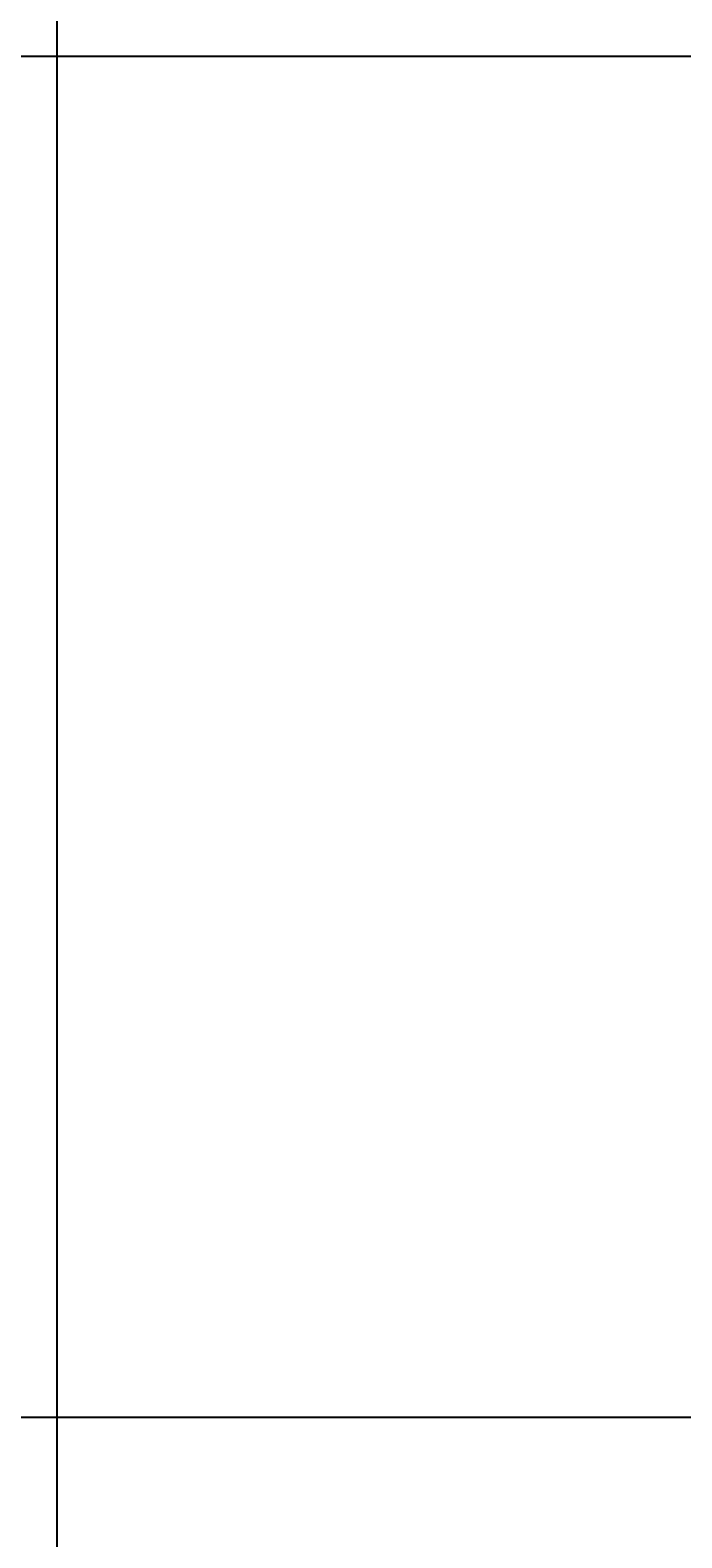
# Model space of a CAD drawing. Units: inches. Extents: x 35362 to 73946, y 43607 to 67532.
# Tile 53 of 134: x 49915 to 50119, y 46091 to 46564. Entities that reach past the tile are written whole.
import ezdxf

# ---------------------------------------------------------------- set-up
doc = ezdxf.new("R2010")
doc.units = ezdxf.units.IN
doc.header["$MEASUREMENT"] = 0
doc.layers.add('A-ANNO-DIMS', color=2, linetype='Continuous', lineweight=18)
doc.styles.get("Standard").update_dxf_attribs({"font": 'arial.ttf'})
doc.dimstyles.get("Standard").update_dxf_attribs({"dimtxt": 0.18, "dimasz": 0.18, "dimexe": 0.18, "dimexo": 0.0625, "dimgap": 0.09, "dimtad": 0, "dimtih": 1, "dimtoh": 1, "dimdec": 4, "dimzin": 0, "dimdsep": 46, "dimtxsty": 'Standard', "dimcen": 0.09, "dimadec": 0, "dimazin": 0, "dimtfac": 1, "dimtdec": 4, "dimtofl": 0, "dimtmove": 0, "dimatfit": 3, "dimfxl": 1, "dimtolj": 1, "dimtzin": 0, "dimarcsym": 0})

# ---------------------------------------------------------------- blocks, each defined once
blk = doc.blocks.new('*D5')
at = {"layer": 'A-ANNO-DIMS', "color": 0, "lineweight": -2, "transparency": 16777216}
for p, q in [((37121.95, 46919.32), (37121.95, 43606.68)), ((69871.5, 45449.83), (69871.5, 43606.68)), ((37122.13, 43606.86), (53496.29, 43606.86)), ((69871.32, 43606.86), (53497.15, 43606.86))]:
    blk.add_line(p, q, dxfattribs=at)
at = {"layer": 'A-ANNO-DIMS', "color": 0, "transparency": 16777216}
for points in [[(37122.13, 43606.89), (37122.13, 43606.83), (37121.95, 43606.86)], [(69871.32, 43606.89), (69871.32, 43606.83), (69871.5, 43606.86)]]:
    blk.add_solid(points, dxfattribs=at)
at = {"layer": 'Defpoints', "color": 0, "transparency": 16777216}
for p in [(37121.95, 46919.38), (69871.5, 45449.89), (69871.5, 43606.86)]:
    blk.add_point(p, dxfattribs=at)
at = {"layer": 'A-ANNO-DIMS', "color": 0, "transparency": 16777216, "insert": (53496.72, 43606.86), "char_height": 0.18, "attachment_point": 5}
blk.add_mtext('\\A1;32750', dxfattribs=at)
blk = doc.blocks.new('*D11')
at = {"layer": 'A-ANNO-DIMS', "color": 0, "lineweight": -2, "transparency": 16777216}
for p, q in [((47978.66, 56028.77), (47978.66, 43606.68)), ((53109.76, 56028.77), (53109.76, 43606.68)), ((47978.84, 43606.86), (50543.87, 43606.86)), ((53109.58, 43606.86), (50544.55, 43606.86))]:
    blk.add_line(p, q, dxfattribs=at)
at = {"layer": 'A-ANNO-DIMS', "color": 0, "transparency": 16777216}
for points in [[(47978.84, 43606.89), (47978.84, 43606.83), (47978.66, 43606.86)], [(53109.58, 43606.89), (53109.58, 43606.83), (53109.76, 43606.86)]]:
    blk.add_solid(points, dxfattribs=at)
at = {"layer": 'Defpoints', "color": 0, "transparency": 16777216}
for p in [(47978.66, 56028.84), (53109.76, 56028.84), (53109.76, 43606.86)]:
    blk.add_point(p, dxfattribs=at)
at = {"layer": 'A-ANNO-DIMS', "color": 0, "transparency": 16777216, "insert": (50544.21, 43606.86), "char_height": 0.18, "attachment_point": 5}
blk.add_mtext('\\A1;5131', dxfattribs=at)
blk = doc.blocks.new('*D13')
at = {"layer": 'A-ANNO-DIMS', "color": 0, "lineweight": -2, "transparency": 16777216}
for p, q in [((48373.49, 51694.02), (48373.49, 43606.68)), ((51029.04, 51694.02), (51029.04, 43606.68)), ((48373.67, 43606.86), (49700.8, 43606.86)), ((51028.86, 43606.86), (49701.73, 43606.86))]:
    blk.add_line(p, q, dxfattribs=at)
at = {"layer": 'A-ANNO-DIMS', "color": 0, "transparency": 16777216}
for points in [[(48373.67, 43606.89), (48373.67, 43606.83), (48373.49, 43606.86)], [(51028.86, 43606.89), (51028.86, 43606.83), (51029.04, 43606.86)]]:
    blk.add_solid(points, dxfattribs=at)
at = {"layer": 'Defpoints', "color": 0, "transparency": 16777216}
for p in [(48373.49, 51694.09), (51029.04, 51694.09), (51029.04, 43606.86)]:
    blk.add_point(p, dxfattribs=at)
at = {"layer": 'A-ANNO-DIMS', "color": 0, "transparency": 16777216, "insert": (49701.27, 43606.86), "char_height": 0.18, "attachment_point": 5}
blk.add_mtext('\\A1;2655.6', dxfattribs=at)
blk = doc.blocks.new('*D17')
at = {"layer": 'A-ANNO-DIMS', "color": 0, "lineweight": -2, "transparency": 16777216}
for p, q in [((49923.31, 61293.22), (49923.31, 43606.68)), ((51913.93, 61293.22), (51913.93, 43606.68)), ((49923.49, 43606.86), (50918.16, 43606.86)), ((51913.75, 43606.86), (50919.07, 43606.86))]:
    blk.add_line(p, q, dxfattribs=at)
at = {"layer": 'A-ANNO-DIMS', "color": 0, "transparency": 16777216}
for points in [[(49923.49, 43606.89), (49923.49, 43606.83), (49923.31, 43606.86)], [(51913.75, 43606.89), (51913.75, 43606.83), (51913.93, 43606.86)]]:
    blk.add_solid(points, dxfattribs=at)
at = {"layer": 'Defpoints', "color": 0, "transparency": 16777216}
for p in [(49923.31, 61293.29), (51913.93, 61293.29), (51913.93, 43606.86)]:
    blk.add_point(p, dxfattribs=at)
at = {"layer": 'A-ANNO-DIMS', "color": 0, "transparency": 16777216, "insert": (50918.62, 43606.86), "char_height": 0.18, "attachment_point": 5}
blk.add_mtext('\\A1;1990.6', dxfattribs=at)
blk = doc.blocks.new('*D67')
at = {"layer": 'A-ANNO-DIMS', "color": 0, "lineweight": -2, "transparency": 16777216}
for p, q in [((56873.54, 53351.53), (35361.77, 53351.53)), ((35361.95, 53351.35), (35361.95, 49400.89)), ((35361.95, 45450.07), (35361.95, 49400.53)), ((53793.58, 45449.89), (35361.77, 45449.89))]:
    blk.add_line(p, q, dxfattribs=at)
at = {"layer": 'A-ANNO-DIMS', "color": 0, "transparency": 16777216}
for points in [[(35361.92, 53351.35), (35361.98, 53351.35), (35361.95, 53351.53)], [(35361.92, 45450.07), (35361.98, 45450.07), (35361.95, 45449.89)]]:
    blk.add_solid(points, dxfattribs=at)
at = {"layer": 'Defpoints', "color": 0, "transparency": 16777216}
for p in [(35361.95, 53351.53), (56873.6, 53351.53), (53793.64, 45449.89)]:
    blk.add_point(p, dxfattribs=at)
at = {"layer": 'A-ANNO-DIMS', "color": 0, "transparency": 16777216, "insert": (35361.95, 49400.71), "char_height": 0.18, "attachment_point": 5}
blk.add_mtext('\\A1;7901.6', dxfattribs=at)
blk = doc.blocks.new('*D76')
at = {"layer": 'A-ANNO-DIMS', "color": 0, "lineweight": -2, "transparency": 16777216}
for p, q in [((54052.84, 46555.29), (35361.77, 46555.29)), ((35361.95, 46555.11), (35361.95, 46342.27)), ((35361.95, 46129.06), (35361.95, 46341.9)), ((53793.58, 46128.88), (35361.77, 46128.88))]:
    blk.add_line(p, q, dxfattribs=at)
at = {"layer": 'A-ANNO-DIMS', "color": 0, "transparency": 16777216}
for points in [[(35361.92, 46555.11), (35361.98, 46555.11), (35361.95, 46555.29)], [(35361.92, 46129.06), (35361.98, 46129.06), (35361.95, 46128.88)]]:
    blk.add_solid(points, dxfattribs=at)
at = {"layer": 'Defpoints', "color": 0, "transparency": 16777216}
for p in [(35361.95, 46555.29), (54052.9, 46555.29), (53793.64, 46128.88)]:
    blk.add_point(p, dxfattribs=at)
at = {"layer": 'A-ANNO-DIMS', "color": 0, "transparency": 16777216, "insert": (35361.95, 46342.09), "char_height": 0.18, "attachment_point": 5}
blk.add_mtext('\\A1;426.4', dxfattribs=at)
blk = doc.blocks.new('*D90')
at = {"layer": 'A-ANNO-DIMS', "color": 0, "lineweight": -2, "transparency": 16777216}
for p, q in [((53707.72, 47291.29), (35361.77, 47291.29)), ((35361.95, 47291.11), (35361.95, 46710.26)), ((35361.95, 46129.06), (35361.95, 46709.9)), ((53793.58, 46128.88), (35361.77, 46128.88))]:
    blk.add_line(p, q, dxfattribs=at)
at = {"layer": 'A-ANNO-DIMS', "color": 0, "transparency": 16777216}
for points in [[(35361.92, 47291.11), (35361.98, 47291.11), (35361.95, 47291.29)], [(35361.92, 46129.06), (35361.98, 46129.06), (35361.95, 46128.88)]]:
    blk.add_solid(points, dxfattribs=at)
at = {"layer": 'Defpoints', "color": 0, "transparency": 16777216}
for p in [(53707.78, 47291.29), (35361.95, 46128.88), (53793.64, 46128.88)]:
    blk.add_point(p, dxfattribs=at)
at = {"layer": 'A-ANNO-DIMS', "color": 0, "transparency": 16777216, "insert": (35361.95, 46710.08), "char_height": 0.18, "attachment_point": 5}
blk.add_mtext('\\A1;1162.4', dxfattribs=at)

msp = doc.modelspace()

# ---------------------------------------------------------------- dimensions: what is measured, and where the dimension line sits
at = {"layer": 'A-ANNO-DIMS'}
for base, p1, p2, override, picture, middle in [((51913.931, 43606.859), (49923.307, 61293.286), (51913.931, 61293.286), {"dimdec": 1, "dimlfac": 1, "dimrnd": 0, "dimzin": 0, "dimdsep": 46, "dimlunit": 2}, '*D17', (50918.619, 43606.859)), ((53109.76, 43606.859), (47978.665, 56028.836), (53109.76, 56028.836), {"dimdec": 0, "dimlfac": 1, "dimrnd": 0, "dimzin": 0, "dimdsep": 46, "dimlunit": 2}, '*D11', (50544.212, 43606.859)), ((51029.043, 43606.859), (48373.492, 51694.087), (51029.043, 51694.087), {"dimdec": 1, "dimlfac": 1, "dimrnd": 0, "dimzin": 0, "dimdsep": 46, "dimlunit": 2}, '*D13', (49701.267, 43606.859)), ((69871.496, 43606.859), (37121.949, 46919.381), (69871.496, 45449.894), {"dimdec": 0, "dimlfac": 1, "dimrnd": 0, "dimzin": 0, "dimdsep": 46, "dimlunit": 2}, '*D5', (53496.723, 43606.859))]:
    dim = msp.add_linear_dim(base=base, p1=p1, p2=p2, dimstyle='Standard', override=override, dxfattribs=at)
    dim.commit()
    dim.dimension.update_dxf_attribs({"geometry": picture, "text_midpoint": middle})
for base, p1, p2, picture, middle in [((35361.949, 53351.529), (53793.638, 45449.894), (56873.602, 53351.529), '*D67', (35361.949, 49400.712)), ((35361.949, 46128.878), (53707.781, 47291.285), (53793.638, 46128.878), '*D90', (35361.949, 46710.081)), ((35361.949, 46555.293), (53793.638, 46128.878), (54052.899, 46555.293), '*D76', (35361.949, 46342.086))]:
    dim = msp.add_linear_dim(base=base, p1=p1, p2=p2, angle=90, dimstyle='Standard', override={"dimdec": 1, "dimlfac": 1, "dimrnd": 0, "dimzin": 0, "dimdsep": 46, "dimlunit": 2}, dxfattribs=at)
    dim.commit()
    dim.dimension.update_dxf_attribs({"geometry": picture, "text_midpoint": middle})

doc.saveas('drawing.dxf')
